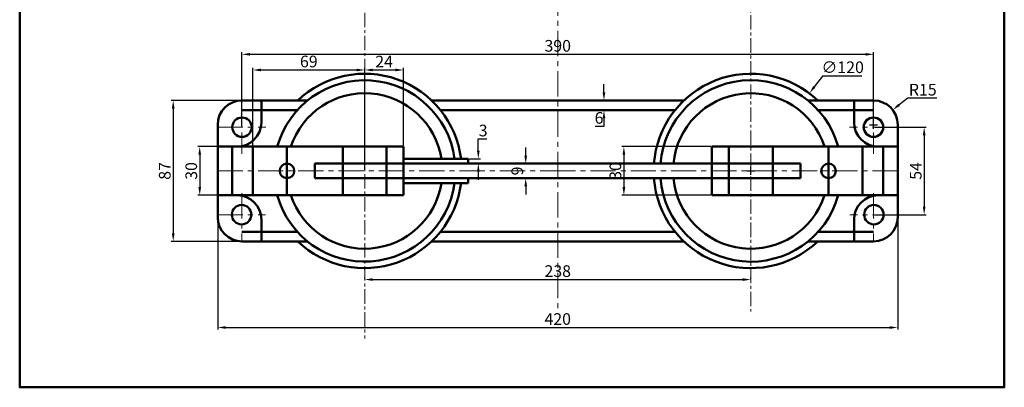
# Model space of a CAD drawing. Units: millimetres. Extents: x -25 to 583, y -116 to 549.
# Tile 1 of 2: x -25 to 583, y -116 to 111. Entities that reach past the tile are written whole.
import ezdxf

# ---------------------------------------------------------------- set-up
doc = ezdxf.new("R2010")
doc.units = ezdxf.units.MM
doc.header["$LTSCALE"] = 0.7
doc.linetypes.add('CENTER', pattern=[50.8, 31.75, -6.35, 6.35, -6.35])
for name, color, linetype, lineweight in [('M-CNTR', 1, 'CENTER', 18), ('M-DIMS', 2, 'Continuous', 25), ('M-OUTL', 7, 'Continuous', 50), ('M-TTLB', 7, 'Continuous', 50)]:
    doc.layers.add(name, color=color, linetype=linetype, lineweight=lineweight)
doc.styles.get("Standard").update_dxf_attribs({"font": 'arial.ttf'})
doc.dimstyles.new('ISO-25', dxfattribs={"dimtxt": 7.2, "dimasz": 5, "dimexe": 1.25, "dimexo": 0.625, "dimtad": 1, "dimtoh": 1, "dimdec": 0, "dimtxsty": 'Standard', "dimcen": 2.5, "dimadec": 0, "dimazin": 0, "dimtfac": 1, "dimtdec": 0, "dimtofl": 0, "dimtmove": 0, "dimatfit": 3, "dimfxl": 1, "dimarcsym": 0})

# ---------------------------------------------------------------- blocks, each defined once
blk = doc.blocks.new('*D34')
at = {"layer": 'Defpoints', "color": 0, "ltscale": 0.7, "transparency": 16777216}
for p in [(462.84, 65.43), (390.52, -30.33)]:
    blk.add_point(p, dxfattribs=at)
at = {"layer": 'M-DIMS', "color": 0, "lineweight": -2, "ltscale": 0.7, "transparency": 16777216}
for p, q in [((470.92, 76.12), (465.86, 69.42)), ((495.26, 76.12), (470.92, 76.12)), ((426.68, 15.05), (426.68, 20.05)), ((424.18, 17.55), (429.18, 17.55))]:
    blk.add_line(p, q, dxfattribs=at)
at = {"layer": 'M-DIMS', "color": 0, "ltscale": 0.7, "transparency": 16777216}
blk.add_solid([(465.19, 69.92), (466.52, 68.92), (462.84, 65.43)], dxfattribs=at)
at = {"layer": 'M-DIMS', "color": 0, "ltscale": 0.7, "transparency": 16777216, "insert": (483.4, 80.62), "char_height": 7.2, "attachment_point": 5}
blk.add_mtext('∅120', dxfattribs=at)
blk = doc.blocks.new('*D36')
at = {"layer": 'Defpoints', "color": 0, "ltscale": 0.7, "transparency": 16777216}
for p in [(287.42, 22.05), (287.42, 13.05), (287.68, 13.05)]:
    blk.add_point(p, dxfattribs=at)
at = {"layer": 'M-DIMS', "color": 0, "lineweight": -2, "ltscale": 0.7, "transparency": 16777216}
for p, q in [((287.68, 27.05), (287.68, 32.05)), ((288.05, 22.05), (288.93, 22.05)), ((288.05, 13.05), (288.93, 13.05)), ((287.68, 8.05), (287.68, 3.05))]:
    blk.add_line(p, q, dxfattribs=at)
at = {"layer": 'M-DIMS', "color": 0, "ltscale": 0.7, "transparency": 16777216}
for points in [[(286.84, 27.05), (288.51, 27.05), (287.68, 22.05)], [(286.84, 8.05), (288.51, 8.05), (287.68, 13.05)]]:
    blk.add_solid(points, dxfattribs=at)
at = {"layer": 'M-DIMS', "color": 0, "ltscale": 0.7, "transparency": 16777216, "insert": (283.38, 17.55), "char_height": 7.2, "attachment_point": 5, "rotation": 90}
blk.add_mtext('9', dxfattribs=at)
blk = doc.blocks.new('*D37')
at = {"layer": 'Defpoints', "color": 0, "ltscale": 0.7, "transparency": 16777216}
for p in [(252.1, 25.05), (252.1, 22.05), (258.4, 22.05)]:
    blk.add_point(p, dxfattribs=at)
at = {"layer": 'M-DIMS', "color": 0, "lineweight": -2, "ltscale": 0.7, "transparency": 16777216}
for p, q in [((258.4, 30.05), (258.4, 37.27)), ((258.4, 37.27), (263.74, 37.27)), ((252.72, 25.05), (259.65, 25.05)), ((252.72, 22.05), (259.65, 22.05)), ((258.4, 17.05), (258.4, 12.05))]:
    blk.add_line(p, q, dxfattribs=at)
at = {"layer": 'M-DIMS', "color": 0, "ltscale": 0.7, "transparency": 16777216}
for points in [[(257.57, 30.05), (259.24, 30.05), (258.4, 25.05)], [(257.57, 17.05), (259.24, 17.05), (258.4, 22.05)]]:
    blk.add_solid(points, dxfattribs=at)
at = {"layer": 'M-DIMS', "color": 0, "ltscale": 0.7, "transparency": 16777216, "insert": (261.38, 41.57), "char_height": 7.2, "attachment_point": 5}
blk.add_mtext('3', dxfattribs=at)
blk = doc.blocks.new('*D38')
at = {"layer": 'Defpoints', "color": 0, "ltscale": 0.7, "transparency": 16777216}
for p in [(97.45, 32.55), (86.36, 2.55), (97.45, 2.55)]:
    blk.add_point(p, dxfattribs=at)
at = {"layer": 'M-DIMS', "color": 0, "lineweight": -2, "ltscale": 0.7, "transparency": 16777216}
for p, q in [((96.83, 32.55), (85.11, 32.55)), ((86.36, 27.55), (86.36, 7.55)), ((96.83, 2.55), (85.11, 2.55))]:
    blk.add_line(p, q, dxfattribs=at)
at = {"layer": 'M-DIMS', "color": 0, "ltscale": 0.7, "transparency": 16777216}
for points in [[(85.53, 27.55), (87.19, 27.55), (86.36, 32.55)], [(85.53, 7.55), (87.19, 7.55), (86.36, 2.55)]]:
    blk.add_solid(points, dxfattribs=at)
at = {"layer": 'M-DIMS', "color": 0, "ltscale": 0.7, "transparency": 16777216, "insert": (82.06, 17.55), "char_height": 7.2, "attachment_point": 5, "rotation": 90}
blk.add_mtext('30', dxfattribs=at)
blk = doc.blocks.new('*D39')
at = {"layer": 'Defpoints', "color": 0, "ltscale": 0.7, "transparency": 16777216}
for p in [(132.7, 61.05), (69.98, -25.95), (132.7, -25.95)]:
    blk.add_point(p, dxfattribs=at)
at = {"layer": 'M-DIMS', "color": 0, "lineweight": -2, "ltscale": 0.7, "transparency": 16777216}
for p, q in [((132.08, 61.05), (68.73, 61.05)), ((69.98, 56.05), (69.98, -20.95)), ((132.08, -25.95), (68.73, -25.95))]:
    blk.add_line(p, q, dxfattribs=at)
at = {"layer": 'M-DIMS', "color": 0, "ltscale": 0.7, "transparency": 16777216}
for points in [[(69.14, 56.05), (70.81, 56.05), (69.98, 61.05)], [(69.14, -20.95), (70.81, -20.95), (69.98, -25.95)]]:
    blk.add_solid(points, dxfattribs=at)
at = {"layer": 'M-DIMS', "color": 0, "ltscale": 0.7, "transparency": 16777216, "insert": (65.68, 17.55), "char_height": 7.2, "attachment_point": 5, "rotation": 90}
blk.add_mtext('87', dxfattribs=at)
blk = doc.blocks.new('*D40')
at = {"layer": 'Defpoints', "color": 0, "ltscale": 0.7, "transparency": 16777216}
for p in [(188.22, -49.5), (426.68, -49.5), (426.68, -49.5)]:
    blk.add_point(p, dxfattribs=at)
at = {"layer": 'M-DIMS', "color": 0, "lineweight": -2, "ltscale": 0.7, "transparency": 16777216}
for p, q in [((188.22, -48.88), (188.22, -48.25)), ((426.68, -48.88), (426.68, -48.25)), ((193.22, -49.5), (421.68, -49.5))]:
    blk.add_line(p, q, dxfattribs=at)
at = {"layer": 'M-DIMS', "color": 0, "ltscale": 0.7, "transparency": 16777216}
for points in [[(193.22, -48.67), (193.22, -50.34), (188.22, -49.5)], [(421.68, -48.67), (421.68, -50.34), (426.68, -49.5)]]:
    blk.add_solid(points, dxfattribs=at)
at = {"layer": 'M-DIMS', "color": 0, "ltscale": 0.7, "transparency": 16777216, "insert": (307.45, -45.2), "char_height": 7.2, "attachment_point": 5}
blk.add_mtext('238', dxfattribs=at)
blk = doc.blocks.new('*D41')
at = {"layer": 'Defpoints', "color": 0, "ltscale": 0.7, "transparency": 16777216}
for p in [(97.45, 17.55), (517.45, 17.55), (517.45, -79.09)]:
    blk.add_point(p, dxfattribs=at)
at = {"layer": 'M-DIMS', "color": 0, "lineweight": -2, "ltscale": 0.7, "transparency": 16777216}
for p, q in [((97.45, 16.93), (97.45, -80.34)), ((517.45, 16.93), (517.45, -80.34)), ((102.45, -79.09), (512.45, -79.09))]:
    blk.add_line(p, q, dxfattribs=at)
at = {"layer": 'M-DIMS', "color": 0, "ltscale": 0.7, "transparency": 16777216}
for points in [[(102.45, -78.26), (102.45, -79.93), (97.45, -79.09)], [(512.45, -78.26), (512.45, -79.93), (517.45, -79.09)]]:
    blk.add_solid(points, dxfattribs=at)
at = {"layer": 'M-DIMS', "color": 0, "ltscale": 0.7, "transparency": 16777216, "insert": (307.45, -74.79), "char_height": 7.2, "attachment_point": 5}
blk.add_mtext('420', dxfattribs=at)
blk = doc.blocks.new('*D42')
at = {"layer": 'Defpoints', "color": 0, "ltscale": 0.7, "transparency": 16777216}
for p in [(502.55, 89.54), (112.35, 44.55), (502.55, 44.55)]:
    blk.add_point(p, dxfattribs=at)
at = {"layer": 'M-DIMS', "color": 0, "lineweight": -2, "ltscale": 0.7, "transparency": 16777216}
for p, q in [((112.35, 45.18), (112.35, 90.79)), ((117.35, 89.54), (497.55, 89.54)), ((502.55, 45.18), (502.55, 90.79))]:
    blk.add_line(p, q, dxfattribs=at)
at = {"layer": 'M-DIMS', "color": 0, "ltscale": 0.7, "transparency": 16777216}
for points in [[(117.35, 90.38), (117.35, 88.71), (112.35, 89.54)], [(497.55, 90.38), (497.55, 88.71), (502.55, 89.54)]]:
    blk.add_solid(points, dxfattribs=at)
at = {"layer": 'M-DIMS', "color": 0, "ltscale": 0.7, "transparency": 16777216, "insert": (307.45, 93.85), "char_height": 7.2, "attachment_point": 5}
blk.add_mtext('390', dxfattribs=at)
blk = doc.blocks.new('*D43')
at = {"layer": 'Defpoints', "color": 0, "ltscale": 0.7, "transparency": 16777216}
for p in [(337.01, 61.05), (335.98, 55.05), (337.01, 55.05)]:
    blk.add_point(p, dxfattribs=at)
at = {"layer": 'M-DIMS', "color": 0, "lineweight": -2, "ltscale": 0.7, "transparency": 16777216}
for p, q in [((335.98, 66.05), (335.98, 71.05)), ((336.38, 61.05), (334.73, 61.05)), ((336.38, 55.05), (334.73, 55.05)), ((335.98, 50.05), (335.98, 45.05)), ((335.98, 45.05), (330.6, 45.05))]:
    blk.add_line(p, q, dxfattribs=at)
at = {"layer": 'M-DIMS', "color": 0, "ltscale": 0.7, "transparency": 16777216}
for points in [[(335.15, 66.05), (336.82, 66.05), (335.98, 61.05)], [(335.15, 50.05), (336.82, 50.05), (335.98, 55.05)]]:
    blk.add_solid(points, dxfattribs=at)
at = {"layer": 'M-DIMS', "color": 0, "ltscale": 0.7, "transparency": 16777216, "insert": (332.98, 49.35), "char_height": 7.2, "attachment_point": 5}
blk.add_mtext('6', dxfattribs=at)
blk = doc.blocks.new('*D44')
at = {"layer": 'Defpoints', "color": 0, "ltscale": 0.7, "transparency": 16777216}
for p in [(402.68, 32.55), (348.3, 2.55), (402.68, 2.55)]:
    blk.add_point(p, dxfattribs=at)
at = {"layer": 'M-DIMS', "color": 0, "lineweight": -2, "ltscale": 0.7, "transparency": 16777216}
for p, q in [((402.06, 32.55), (347.05, 32.55)), ((348.3, 27.55), (348.3, 7.55)), ((402.06, 2.55), (347.05, 2.55))]:
    blk.add_line(p, q, dxfattribs=at)
at = {"layer": 'M-DIMS', "color": 0, "ltscale": 0.7, "transparency": 16777216}
for points in [[(347.46, 27.55), (349.13, 27.55), (348.3, 32.55)], [(347.46, 7.55), (349.13, 7.55), (348.3, 2.55)]]:
    blk.add_solid(points, dxfattribs=at)
at = {"layer": 'M-DIMS', "color": 0, "ltscale": 0.7, "transparency": 16777216, "insert": (343.99, 17.55), "char_height": 7.2, "attachment_point": 5, "rotation": 90}
blk.add_mtext('30', dxfattribs=at)
blk = doc.blocks.new('*D45')
at = {"layer": 'Defpoints', "color": 0, "ltscale": 0.7, "transparency": 16777216}
for p in [(502.55, 44.55), (502.45, -9.45), (533.75, -9.45)]:
    blk.add_point(p, dxfattribs=at)
at = {"layer": 'M-DIMS', "color": 0, "lineweight": -2, "ltscale": 0.7, "transparency": 16777216}
for p, q in [((503.18, 44.55), (535, 44.55)), ((533.75, 39.55), (533.75, -4.45)), ((503.08, -9.45), (535, -9.45))]:
    blk.add_line(p, q, dxfattribs=at)
at = {"layer": 'M-DIMS', "color": 0, "ltscale": 0.7, "transparency": 16777216}
for points in [[(532.91, 39.55), (534.58, 39.55), (533.75, 44.55)], [(532.91, -4.45), (534.58, -4.45), (533.75, -9.45)]]:
    blk.add_solid(points, dxfattribs=at)
at = {"layer": 'M-DIMS', "color": 0, "ltscale": 0.7, "transparency": 16777216, "insert": (529.46, 17.55), "char_height": 7.2, "attachment_point": 5, "rotation": 90}
blk.add_mtext('54', dxfattribs=at)
blk = doc.blocks.new('*D46')
at = {"layer": 'Defpoints', "color": 0, "ltscale": 0.7, "transparency": 16777216}
for p in [(514.3, 55.25), (502.45, 46.05)]:
    blk.add_point(p, dxfattribs=at)
at = {"layer": 'M-DIMS', "color": 0, "lineweight": -2, "ltscale": 0.7, "transparency": 16777216}
for p, q in [((523.62, 62.48), (518.25, 58.31)), ((541.5, 62.48), (523.62, 62.48)), ((499.95, 46.05), (504.95, 46.05)), ((502.45, 43.55), (502.45, 48.55))]:
    blk.add_line(p, q, dxfattribs=at)
at = {"layer": 'M-DIMS', "color": 0, "ltscale": 0.7, "transparency": 16777216}
blk.add_solid([(517.74, 58.97), (518.76, 57.66), (514.3, 55.25)], dxfattribs=at)
at = {"layer": 'M-DIMS', "color": 0, "ltscale": 0.7, "transparency": 16777216, "insert": (532.87, 66.78), "char_height": 7.2, "attachment_point": 5}
blk.add_mtext('R15', dxfattribs=at)
blk = doc.blocks.new('*D47')
at = {"layer": 'Defpoints', "color": 0, "ltscale": 0.7, "transparency": 16777216}
for p in [(188.22, 79.88), (119.22, 17.55), (188.22, 17.55)]:
    blk.add_point(p, dxfattribs=at)
at = {"layer": 'M-DIMS', "color": 0, "lineweight": -2, "ltscale": 0.7, "transparency": 16777216}
for p, q in [((119.22, 18.18), (119.22, 81.13)), ((124.22, 79.88), (183.22, 79.88)), ((188.22, 18.18), (188.22, 81.13))]:
    blk.add_line(p, q, dxfattribs=at)
at = {"layer": 'M-DIMS', "color": 0, "ltscale": 0.7, "transparency": 16777216}
for points in [[(124.22, 80.71), (124.22, 79.04), (119.22, 79.88)], [(183.22, 80.71), (183.22, 79.04), (188.22, 79.88)]]:
    blk.add_solid(points, dxfattribs=at)
at = {"layer": 'M-DIMS', "color": 0, "ltscale": 0.7, "transparency": 16777216, "insert": (153.72, 84.18), "char_height": 7.2, "attachment_point": 5}
blk.add_mtext('69', dxfattribs=at)
blk = doc.blocks.new('*D48')
at = {"layer": 'Defpoints', "color": 0, "ltscale": 0.7, "transparency": 16777216}
for p in [(212.22, 79.88), (188.22, 32.55), (212.22, 32.55)]:
    blk.add_point(p, dxfattribs=at)
at = {"layer": 'M-DIMS', "color": 0, "lineweight": -2, "ltscale": 0.7, "transparency": 16777216}
for p, q in [((188.22, 33.18), (188.22, 81.13)), ((193.22, 79.88), (207.22, 79.88)), ((212.22, 33.18), (212.22, 81.13))]:
    blk.add_line(p, q, dxfattribs=at)
at = {"layer": 'M-DIMS', "color": 0, "ltscale": 0.7, "transparency": 16777216}
for points in [[(193.22, 80.71), (193.22, 79.04), (188.22, 79.88)], [(207.22, 80.71), (207.22, 79.04), (212.22, 79.88)]]:
    blk.add_solid(points, dxfattribs=at)
at = {"layer": 'M-DIMS', "color": 0, "ltscale": 0.7, "transparency": 16777216, "insert": (200.22, 84.12), "char_height": 7.2, "attachment_point": 5}
blk.add_mtext('24', dxfattribs=at)

msp = doc.modelspace()

# ---------------------------------------------------------------- linework, layer by layer
at = {"layer": 'M-CNTR', "ltscale": 0.4}
for p, q in [((188.22, 413.89), (188.22, -85.81)), ((426.68, 412.37), (426.68, -69.19))]:
    msp.add_line(p, q, dxfattribs=at)
at = {"layer": 'M-CNTR', "ltscale": 0.7}
for p, q in [((307.45, 128.89), (307.45, -67.34)), ((112.45, 66.14), (112.45, 28.05)), ((502.45, 66.14), (502.45, 28.05)), ((97.45, 44.55), (127.24, 44.55)), ((517.45, 44.55), (487.66, 44.55)), ((97.45, 17.55), (307.45, 17.55)), ((517.45, 17.55), (307.45, 17.55)), ((112.45, 3.8), (112.45, -25.95)), ((502.45, 3.8), (502.45, -25.95)), ((97.45, -9.45), (126.98, -9.45)), ((517.45, -9.45), (487.92, -9.45))]:
    msp.add_line(p, q, dxfattribs=at)
at = {"layer": 'M-OUTL', "ltscale": 0.7}
for p, q in [((112.45, 61.05), (152.95, 61.05)), ((124.45, 61.05), (124.45, 47.55)), ((229.55, 61.05), (307.45, 61.05)), ((385.36, 61.05), (307.45, 61.05)), ((502.45, 61.05), (461.95, 61.05)), ((490.45, 61.05), (490.45, 47.55)), ((112.45, 55.05), (146.63, 55.05)), ((235.06, 55.05), (307.45, 55.05)), ((379.84, 55.05), (307.45, 55.05)), ((502.45, 55.05), (468.27, 55.05)), ((97.45, 46.05), (97.45, -10.95)), ((517.45, 46.05), (517.45, -10.95)), ((97.45, 32.55), (109.45, 32.55)), ((106.45, 32.55), (106.45, 2.55)), ((109.45, 32.55), (212.22, 32.55)), ((119.22, 32.55), (119.22, 2.55)), ((140.22, 32.55), (140.22, 2.55)), ((174.72, 32.55), (174.72, 2.55)), ((201.72, 32.55), (201.72, 2.55)), ((212.22, 2.55), (212.22, 32.55)), ((505.45, 32.55), (402.68, 32.55)), ((402.68, 2.55), (402.68, 32.55)), ((413.18, 32.55), (413.18, 2.55)), ((440.18, 32.55), (440.18, 2.55)), ((474.68, 32.55), (474.68, 2.55)), ((495.68, 32.55), (495.68, 2.55)), ((517.45, 32.55), (505.45, 32.55)), ((508.45, 32.55), (508.45, 2.55)), ((212.22, 25.05), (252.1, 25.05)), ((252.1, 25.05), (252.1, 22.05)), ((157.45, 22.05), (157.45, 13.05)), ((157.45, 22.05), (307.45, 22.05)), ((457.45, 22.05), (307.45, 22.05)), ((457.45, 22.05), (457.45, 13.05)), ((157.45, 13.05), (307.45, 13.05)), ((252.1, 13.05), (252.1, 10.05)), ((457.45, 13.05), (307.45, 13.05)), ((212.22, 10.05), (252.1, 10.05)), ((97.45, 2.55), (109.45, 2.55)), ((109.45, 2.55), (212.22, 2.55)), ((505.45, 2.55), (402.68, 2.55)), ((517.45, 2.55), (505.45, 2.55)), ((124.45, -12.45), (124.45, -25.95)), ((490.45, -12.45), (490.45, -25.95)), ((112.45, -19.95), (146.63, -19.95)), ((235.06, -19.95), (307.45, -19.95)), ((379.84, -19.95), (307.45, -19.95)), ((502.45, -19.95), (468.27, -19.95)), ((112.45, -25.95), (152.95, -25.95)), ((229.55, -25.95), (307.45, -25.95)), ((385.36, -25.95), (307.45, -25.95)), ((502.45, -25.95), (461.95, -25.95))]:
    msp.add_line(p, q, dxfattribs=at)
for centre, radius in [((112.45, 44.55), 6), ((502.45, 44.55), 6), ((140.22, 17.55), 4.5), ((474.68, 17.55), 4.5), ((112.21, -9.45), 6), ((502.69, -9.45), 6)]:
    msp.add_circle(centre, radius, dxfattribs=at)
for centre, radius, start, end in [((188.22, 17.55), 56, 7.69667, 164.46321), ((188.22, 17.55), 60, 7.18076, 133.53115), ((426.68, 17.55), 60, 46.46885, 175.69878), ((426.68, 17.55), 56, 15.53679, 175.39091), ((112.45, 46.05), 15, 90, 180), ((188.22, 17.55), 48, 8.9893, 161.79004), ((426.68, 17.55), 48, 18.20996, 174.62062), ((502.45, 46.05), 15, 360, 90), ((109.45, 47.55), 15, 270, 0), ((505.45, 47.55), 15, 180, 270), ((426.68, 17.55), 60, 184.30122, 313.53115), ((426.68, 17.55), 56, 184.60909, 344.46321), ((426.68, 17.55), 48, 185.37938, 341.79004), ((188.22, 17.55), 56, 195.53679, 352.30333), ((188.22, 17.55), 48, 198.20996, 351.0107), ((188.22, 17.55), 60, 226.46885, 352.81924), ((109.45, -12.45), 15, 0, 90), ((505.45, -12.45), 15, 90, 180), ((112.45, -10.95), 15, 180, 270), ((502.45, -10.95), 15, 270, 360)]:
    msp.add_arc(centre, radius, start, end, dxfattribs=at)
at = {"layer": 'M-TTLB', "ltscale": 0.7}
msp.add_lwpolyline([(-24.83, 548.59), (583.23, 548.59), (583.23, -116), (-24.83, -116)], close=True, dxfattribs=at)

# ---------------------------------------------------------------- dimensions: what is measured, and where the dimension line sits
at = {"layer": 'M-DIMS', "ltscale": 0.7}
for base, p1, p2, picture, middle in [((502.55, 89.54), (112.35, 44.55), (502.55, 44.55), '*D42', (307.45, 93.85)), ((188.22, 79.88), (119.22, 17.55), (188.22, 17.55), '*D47', (153.72, 84.18)), ((212.22, 79.88), (188.22, 32.55), (212.22, 32.55), '*D48', (200.22, 84.12)), ((517.45, -79.09), (97.45, 17.55), (517.45, 17.55), '*D41', (307.45, -74.79)), ((426.68, -49.5), (188.22, -49.5), (426.68, -49.5), '*D40', (307.45, -45.2))]:
    dim = msp.add_linear_dim(base=base, p1=p1, p2=p2, dimstyle='ISO-25', override={"dimclrd": 0, "dimclre": 0, "dimclrt": 0}, dxfattribs=at)
    dim.commit()
    dim.dimension.update_dxf_attribs({"geometry": picture, "text_midpoint": middle})
dim = msp.add_diameter_dim_2p(p1=(390.52, -30.33), p2=(462.84, 65.43), dimstyle='ISO-25', override={"dimclrd": 0, "dimclre": 0, "dimclrt": 0}, dxfattribs=at)
dim.commit()
dim.dimension.update_dxf_attribs({"geometry": '*D34', "text_midpoint": (483.4, 76.12), "dimtype": 163})
for base, p1, p2, picture, middle in [((335.98, 55.05), (337.01, 61.05), (337.01, 55.05), '*D43', (332.98, 49.35)), ((69.98, -25.95), (132.7, 61.05), (132.7, -25.95), '*D39', (65.68, 17.55)), ((533.75, -9.45), (502.55, 44.55), (502.45, -9.45), '*D45', (529.46, 17.55)), ((86.36, 2.55), (97.45, 32.55), (97.45, 2.55), '*D38', (82.06, 17.55)), ((287.68, 13.05), (287.42, 22.05), (287.42, 13.05), '*D36', (283.38, 17.55)), ((348.3, 2.55), (402.68, 32.55), (402.68, 2.55), '*D44', (343.99, 17.55))]:
    dim = msp.add_linear_dim(base=base, p1=p1, p2=p2, angle=90, dimstyle='ISO-25', override={"dimclrd": 0, "dimclre": 0, "dimclrt": 0}, dxfattribs=at)
    dim.commit()
    dim.dimension.update_dxf_attribs({"geometry": picture, "text_midpoint": middle})
dim = msp.add_radius_dim(center=(502.45, 46.05), mpoint=(514.3, 55.25), dimstyle='ISO-25', override={"dimclrd": 0, "dimclre": 0, "dimclrt": 0}, dxfattribs=at)
dim.commit()
dim.dimension.update_dxf_attribs({"geometry": '*D46', "text_midpoint": (532.87, 62.48), "dimtype": 164})
dim = msp.add_linear_dim(base=(258.4, 22.05), p1=(252.1, 25.05), p2=(252.1, 22.05), angle=90, dimstyle='ISO-25', override={"dimclrd": 0, "dimclre": 0, "dimclrt": 0}, dxfattribs=at)
dim.commit()
dim.dimension.update_dxf_attribs({"geometry": '*D37', "text_midpoint": (261.38, 37.27), "dimtype": 160})

doc.saveas('drawing.dxf')
